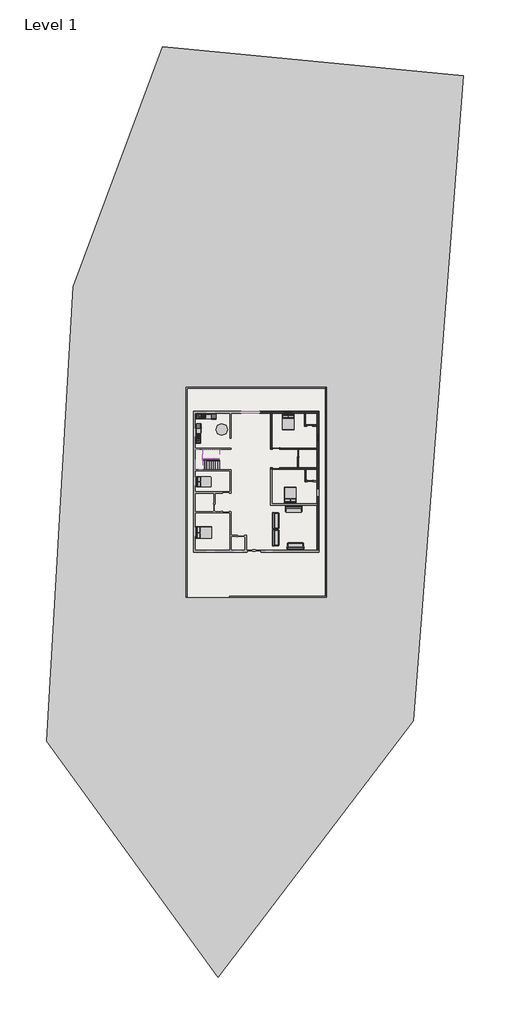
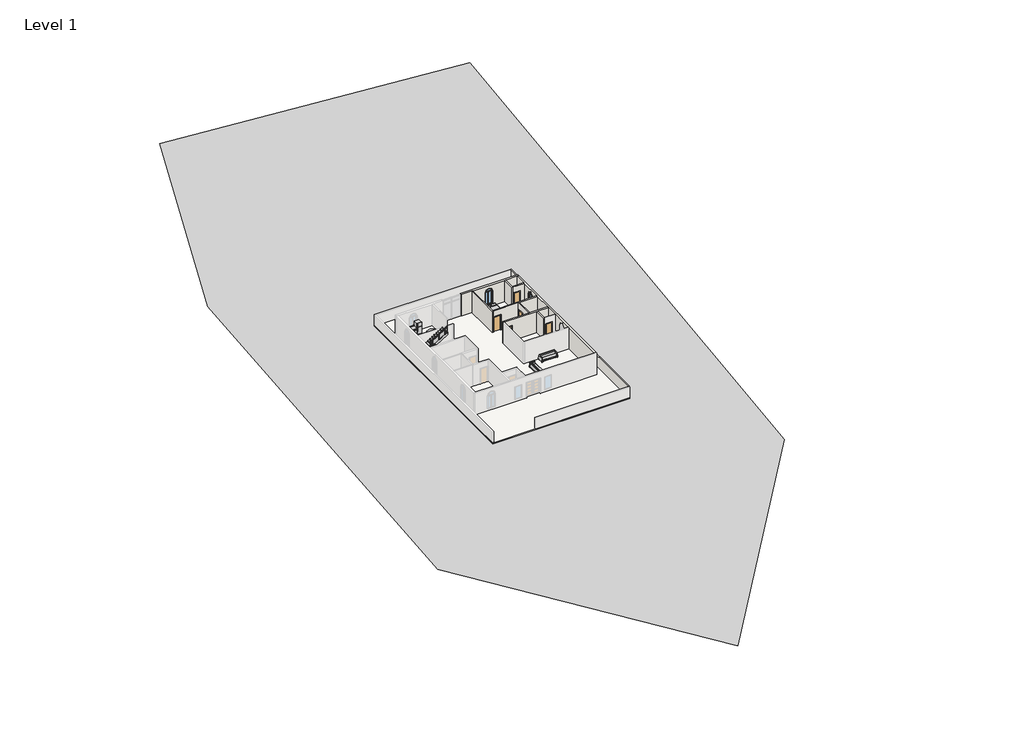
# One storey, part 2 of 2: 11 furniture elements, 10 walls, 9 proxies, 5 doors, 3 members, 2 flow terminals, 2 slabs, 2 stair flights, 3 other elements.
"""IFC4 building model written with IfcOpenShell, lengths in millimetres."""

from ifc_helpers import new_model, si_unit, frame, origin, place, context, project, spatial, polyline, circle_curve, outline, extrude, faceted_brep, triangles, transform, mapped, element, save
from ifc_brep_helpers import plane_surface, revolved_surface, advanced_brep
from components import proxy_a6faaae8, proxy_45b28599, kitchenette_medium_kitchenette_medium_844211aa, proxy_c523a7b7, single_flush_2_5_e2b13fe9, door_686f89d2, door_16372e1c, flow_terminal_871c2e40, furniture_c8abb964, furniture_1d2926bd, furniture_c6510c7c, furniture_aff9b2fb, furniture_bbcc68ce, non_monolithic_landing_a6573d81, stair_flight_969e3d78, stair_flight_057ca7f5, window_e7489165

model = new_model("IFC4")

# Units and contexts
model_context = context("Model", 3, world=origin())
ifc_project = project(units=[si_unit("LENGTHUNIT", "METRE", prefix="MILLI")], contexts=[model_context])

# Site, building, storey
site = spatial("IfcSite", under=ifc_project)
building = spatial("IfcBuilding", under=site)
storey = spatial("IfcBuildingStorey", under=building, Name="Level 1", Elevation=0.0)

# Proxies
placement = place(None, origin())
element("IfcBuildingElementProxy", 1, Name="Building Element Proxy", at=placement, inside=storey, context=model_context, shape_type="Tessellation", body=[
    triangles([(-13362.1157867, 60522.4871704, -152.4), (26139.3672729, 56668.527063, -152.4), (19592.1599304, -27911.1312195, -152.4), (-6089.9317657, -61567.0048096, -152.4), (-28593.0151794, -30596.776593, -152.4), (-25067.8233765, 29048.3780823, -152.4)], [[6, 2, 1], [3, 6, 5], [3, 2, 6], [3, 5, 4]], closed=False),
])
proxy_shape = proxy_a6faaae8(model_context)
element("IfcBuildingElementProxy", 2, Name="Cook Top-4 Unit2 : 22\" x 20\"", ObjectType="Cook Top-4 Unit2 : 22\" x 20\"", at=placement, inside=storey, context=model_context, shape_type="MappedRepresentation", body=[
    mapped(proxy_shape, transform((-8593.9791271, 12037.2953048, 0.0), x_axis=(1.0, 0.0, 0.0), y_axis=(0.0, 1.0, 0.0), z_axis=(0.0, 0.0, 1.0))),
])
element("IfcBuildingElementProxy", 3, Name="Cook Top-4 Unit2 : 22\" x 20\"", ObjectType="Cook Top-4 Unit2 : 22\" x 20\"", at=placement, inside=storey, context=model_context, shape_type="MappedRepresentation", body=[
    mapped(proxy_shape, transform((-8670.1791271, 8836.8953048, 0.0), x_axis=(0.0, 1.0000000000000002, 0.0), y_axis=(-1.0000000000000002, 0.0, 0.0), z_axis=(0.0, 0.0, 1.0))),
])
proxy_2_shape = proxy_45b28599(model_context)
element("IfcBuildingElementProxy", 4, Name="Dishwasher : 24\" x 24\" x 34\"", ObjectType="Dishwasher : 24\" x 24\" x 34\"", at=placement, inside=storey, context=model_context, shape_type="MappedRepresentation", body=[
    mapped(proxy_2_shape, transform((-7642.7965956, 11745.44574, 0.0), x_axis=(1.0, 0.0, 0.0), y_axis=(0.0, 1.0, 0.0), z_axis=(0.0, 0.0, 1.0))),
])
element("IfcBuildingElementProxy", 5, Name="Dishwasher : 24\" x 24\" x 34\"", ObjectType="Dishwasher : 24\" x 24\" x 34\"", at=placement, inside=storey, context=model_context, shape_type="MappedRepresentation", body=[
    mapped(proxy_2_shape, transform((-8378.3295623, 9788.0778363, 0.0), x_axis=(0.0, 1.0000000000000002, 0.0), y_axis=(-1.0000000000000002, 0.0, 0.0), z_axis=(0.0, 0.0, 1.0))),
])
kitchenette_medium_kitchenette_medium_shape = kitchenette_medium_kitchenette_medium_844211aa(model_context)
element("IfcBuildingElementProxy", 6, Name="Kitchenette - Medium : Kitchenette - Medium", ObjectType="Kitchenette - Medium : Kitchenette - Medium", at=placement, inside=storey, context=model_context, shape_type="MappedRepresentation", body=[
    mapped(kitchenette_medium_kitchenette_medium_shape, transform((-8269.816832, 12342.0953048, 0.0), x_axis=(1.0, 0.0, 0.0), y_axis=(0.0, 1.0, 0.0), z_axis=(0.0, 0.0, 1.0))),
])
element("IfcBuildingElementProxy", 7, Name="Kitchenette - Medium : Kitchenette - Medium", ObjectType="Kitchenette - Medium : Kitchenette - Medium", at=placement, inside=storey, context=model_context, shape_type="MappedRepresentation", body=[
    mapped(kitchenette_medium_kitchenette_medium_shape, transform((-8974.9791271, 9161.0575999, 0.0), x_axis=(0.0, 1.0000000000000002, 0.0), y_axis=(-1.0000000000000002, 0.0, 0.0), z_axis=(0.0, 0.0, 1.0))),
])
proxy_3_shape = proxy_c523a7b7(model_context)
element("IfcBuildingElementProxy", 8, Name="Refrigerator : 24\" x 25\" LH", ObjectType="Refrigerator : 24\" x 25\" LH", at=placement, inside=storey, context=model_context, shape_type="MappedRepresentation", body=[
    mapped(proxy_3_shape, transform((-6657.2291271, 11991.6463333, 0.0), x_axis=(1.0, 0.0, 0.0), y_axis=(0.0, 1.0, 0.0), z_axis=(0.0, 0.0, 1.0))),
])
element("IfcBuildingElementProxy", 9, Name="Refrigerator : 24\" x 25\" LH", ObjectType="Refrigerator : 24\" x 25\" LH", at=placement, inside=storey, context=model_context, shape_type="MappedRepresentation", body=[
    mapped(proxy_3_shape, transform((-8624.5301556, 10773.6453048, 0.0), x_axis=(0.0, 1.0000000000000002, 0.0), y_axis=(-1.0000000000000002, 0.0, 0.0), z_axis=(0.0, 0.0, 1.0))),
])

# Doors
single_flush_2_5_shape = single_flush_2_5_e2b13fe9(model_context)
element("IfcDoor", 10, ObjectType="Single-Flush : 2.5'", at=placement, inside=storey, context=model_context, shape_type="MappedRepresentation", body=[
    mapped(single_flush_2_5_shape, transform((6023.7208729, 3515.5953048, 0.0), x_axis=(-1.0, 0.0, 0.0), y_axis=(0.0, -1.0, 0.0), z_axis=(0.0, 0.0, 1.0))),
])
element("IfcDoor", 11, ObjectType="Single-Flush : 2.5'", at=placement, inside=storey, context=model_context, shape_type="MappedRepresentation", body=[
    mapped(single_flush_2_5_shape, transform((5947.5208729, 10830.7953048, 0.0), x_axis=(-1.0, 0.0, 0.0), y_axis=(0.0, -1.0, 0.0), z_axis=(0.0, 0.0, 1.0))),
])
door_shape = door_686f89d2(model_context)
element("IfcDoor", 12, ObjectType="Single-Flush : 36\" x 84\"", at=placement, inside=storey, context=model_context, shape_type="MappedRepresentation", body=[
    mapped(door_shape, transform((1527.9208729, 7782.7953048, 0.0), x_axis=(-1.0, 0.0, 0.0), y_axis=(0.0, -1.0, 0.0), z_axis=(0.0, 0.0, 1.0))),
])
element("IfcDoor", 13, ObjectType="Single-Flush : 36\" x 84\"", at=placement, inside=storey, context=model_context, shape_type="MappedRepresentation", body=[
    mapped(door_shape, transform((4423.5208729, 7173.1953048, 0.0), x_axis=(0.0, 1.0, 0.0), y_axis=(-1.0, 0.0, 0.0), z_axis=(0.0, 0.0, 1.0))),
])
door_2_shape = door_16372e1c(model_context)
element("IfcDoor", 14, ObjectType="Single-Flush : 36\" x 84\"", at=placement, inside=storey, context=model_context, shape_type="MappedRepresentation", body=[
    mapped(door_2_shape, transform((1527.9208729, 5191.9953048, 0.0), x_axis=(-1.0, 0.0, 0.0), y_axis=(0.0, -1.0, 0.0), z_axis=(0.0, 0.0, 1.0))),
])

# Flow terminals
flow_terminal_shape = flow_terminal_871c2e40(model_context)
element("IfcFlowTerminal", 15, ObjectType="Sink Kitchen-Island : 18\" x 18\"", at=placement, inside=storey, context=model_context, shape_type="MappedRepresentation", body=[
    mapped(flow_terminal_shape, transform((-7936.5683676, 12034.9499037, -14.4), x_axis=(1.0, 0.0, 0.0), y_axis=(0.0, 1.0, 0.0), z_axis=(0.0, 0.0, 1.0))),
])
element("IfcFlowTerminal", 16, ObjectType="Sink Kitchen-Island : 18\" x 18\"", at=placement, inside=storey, context=model_context, shape_type="MappedRepresentation", body=[
    mapped(flow_terminal_shape, transform((-8667.833726, 9494.3060642, -14.4), x_axis=(0.0, 1.0000000000000002, 0.0), y_axis=(-1.0000000000000002, 0.0, 0.0), z_axis=(0.0, 0.0, 1.0))),
])

# Furniture
furniture_shape = furniture_c8abb964(model_context)
element("IfcFurniture", 17, ObjectType="Bed-Box : Double 53\" x 74\"", at=placement, inside=storey, context=model_context, shape_type="MappedRepresentation", body=[
    mapped(furniture_shape, transform((-8168.0086353, 3100.2428458, 0.0), x_axis=(0.0, 1.0, 0.0), y_axis=(-1.0, 0.0, 0.0), z_axis=(0.0, 0.0, 1.0))),
])
furniture_2_shape = furniture_1d2926bd(model_context)
element("IfcFurniture", 18, ObjectType="Bed-Box : Queen 60\" x 79\"", at=placement, inside=storey, context=model_context, shape_type="MappedRepresentation", body=[
    mapped(furniture_2_shape, transform((-8168.0086353, -3571.0046952, 0.0), x_axis=(0.0, 1.0000000000000002, 0.0), y_axis=(-1.0000000000000002, 0.0, 0.0), z_axis=(0.0, 0.0, 1.0))),
])
element("IfcFurniture", 19, ObjectType="Bed-Box : Queen 60\" x 79\"", at=placement, inside=storey, context=model_context, shape_type="MappedRepresentation", body=[
    mapped(furniture_2_shape, transform((3759.3733319, 1477.7657966, 0.0), x_axis=(-1.0, 0.0, 0.0), y_axis=(0.0, -1.0, 0.0), z_axis=(0.0, 0.0, 1.0))),
])
element("IfcFurniture", 20, ObjectType="Bed-Box : Queen 60\" x 79\"", at=placement, inside=storey, context=model_context, shape_type="MappedRepresentation", body=[
    mapped(furniture_2_shape, transform((2801.6684139, 11535.124813, 0.0), x_axis=(1.0000000000000002, 0.0, 0.0), y_axis=(0.0, 1.0000000000000002, 0.0), z_axis=(0.0, 0.0, 1.0))),
])
furniture_3_shape = furniture_c6510c7c(model_context)
element("IfcFurniture", 21, ObjectType="Counter Top w Sink Hole : 24\" Depth", at=placement, inside=storey, context=model_context, shape_type="MappedRepresentation", body=[
    mapped(furniture_3_shape, transform((-7736.416832, 12342.0953048, -14.4), x_axis=(1.0, 0.0, 0.0), y_axis=(0.0, 1.0, 0.0), z_axis=(0.0, 0.0, 1.0))),
])
element("IfcFurniture", 22, ObjectType="Counter Top w Sink Hole : 24\" Depth", at=placement, inside=storey, context=model_context, shape_type="MappedRepresentation", body=[
    mapped(furniture_3_shape, transform((-8974.9791271, 9694.4575999, -14.4), x_axis=(0.0, 1.0000000000000002, 0.0), y_axis=(-1.0000000000000002, 0.0, 0.0), z_axis=(0.0, 0.0, 1.0))),
])
furniture_4_shape = furniture_aff9b2fb(model_context)
element("IfcFurniture", 23, ObjectType="Sofa-Pensi : 84\"", at=placement, inside=storey, context=model_context, shape_type="MappedRepresentation", body=[
    mapped(furniture_4_shape, transform((3586.1146229, -419.1145313, 0.0), x_axis=(1.0, 0.0, 0.0), y_axis=(0.0, 1.0, 0.0), z_axis=(0.0, 0.0, 1.0))),
])
element("IfcFurniture", 24, ObjectType="Sofa-Pensi : 84\"", at=placement, inside=storey, context=model_context, shape_type="MappedRepresentation", body=[
    mapped(furniture_4_shape, transform((1754.230709, -1944.6109452, 0.0), x_axis=(0.0, 1.0000000000000002, 0.0), y_axis=(-1.0000000000000002, 0.0, 0.0), z_axis=(0.0, 0.0, 1.0))),
])
element("IfcFurniture", 25, ObjectType="Sofa-Pensi : 84\"", at=placement, inside=storey, context=model_context, shape_type="MappedRepresentation", body=[
    mapped(furniture_4_shape, transform((4371.9271229, -4728.9948591, 0.0), x_axis=(-1.0000000000000004, 0.0, 0.0), y_axis=(0.0, -1.0000000000000004, 0.0), z_axis=(0.0, 0.0, 1.0))),
])
element("IfcFurniture", 26, ObjectType="Sofa-Pensi : 84\"", at=placement, inside=storey, context=model_context, shape_type="MappedRepresentation", body=[
    mapped(furniture_4_shape, transform((1754.230709, -4179.8109452, 0.0), x_axis=(0.0, 1.0000000000000009, 0.0), y_axis=(-1.0000000000000009, 0.0, 0.0), z_axis=(0.0, 0.0, 1.0))),
])
furniture_5_shape = furniture_bbcc68ce(model_context)
element("IfcFurniture", 27, ObjectType="Table-Dining Round w Chairs : 36\" Diameter", at=placement, inside=storey, context=model_context, shape_type="MappedRepresentation", body=[
    mapped(furniture_5_shape, transform((-5687.7610943, 10482.2739933, 0.0), x_axis=(1.0, 0.0, 0.0), y_axis=(0.0, 1.0, 0.0), z_axis=(0.0, 0.0, 1.0))),
])

# Members
element("IfcMember", 28, ObjectType="Stringer - 2\" Width", at=placement, inside=storey, context=model_context, shape_type="SweptSolid", body=[
    extrude(outline(polyline([(0.0, -5888.8791271), (215.0106437, -5888.8791271), (1605.083371, -8073.2791271), (1243.8010268, -8073.2791271), (0.0, -6118.7346564), (0.0, -5888.8791271)])), frame((0.0, 6233.3953048, 0.0), z_axis=(0.0, 1.0, 0.0), x_axis=(0.0, 0.0, 1.0)), (0.0, 0.0, 1.0), 50.8),
])
element("IfcMember", 29, ObjectType="Stringer - 2\" Width", at=placement, inside=storey, context=model_context, shape_type="SweptSolid", body=[
    extrude(outline(polyline([(1815.2106437, -8124.0791271), (1453.9282995, -8124.0791271), (2876.3282995, -5888.8791271), (3237.6106437, -5888.8791271), (1815.2106437, -8124.0791271)])), frame((0.0, 6411.1953048, 0.0), z_axis=(0.0, 1.0, 0.0), x_axis=(0.0, 0.0, 1.0)), (0.0, 0.0, 1.0), 50.8),
])
element("IfcMember", 30, ObjectType="Stringer - 2\" Width", at=placement, inside=storey, context=model_context, shape_type="SweptSolid", body=[
    extrude(outline(polyline([(-8073.2791271, 6233.3953048), (-8124.0791271, 6233.3953048), (-8124.0791271, 6411.1953048), (-8073.2791271, 6411.1953048), (-8073.2791271, 6233.3953048)])), frame((0.0, 0.0, 1371.6), z_axis=(0.0, 0.0, 1.0), x_axis=(1.0, 0.0, 0.0)), (0.0, 0.0, 1.0), 304.8),
])

# Railing
element("IfcRailing", 31, ObjectType="Glass Panel - Bottom Fill", at=placement, inside=storey, context=model_context, shape_type="SolidModel", body=[
    faceted_brep([(-5888.8791271, 6182.5953048, 1092.2), (-5888.8791271, 6182.5953048, 1031.986276), (-5888.8791271, 6233.3953048, 1031.986276), (-5888.8791271, 6233.3953048, 1092.2), (-8047.8791271, 6182.5953048, 2466.1090909), (-8098.6791271, 6182.5953048, 2438.2226396), (-8098.6791271, 6233.3953048, 2438.2226396), (-8047.8791271, 6233.3953048, 2466.1090909), (-8174.8791271, 6309.5953048, 2463.8), (-8174.8791271, 6309.5953048, 2514.6), (-8174.8791271, 6385.7953048, 2514.6), (-8174.8791271, 6436.5953048, 2463.8), (-8124.0791271, 6309.5953048, 2463.8), (-8124.0791271, 6436.5953048, 2463.8), (-8124.0791271, 6309.5953048, 2514.6), (-8124.0791271, 6385.7953048, 2514.6), (-8174.8791271, 6385.7953048, 2740.8909091), (-8174.8791271, 6436.5953048, 2690.0909091), (-8124.0791271, 6436.5953048, 2690.0909091), (-8124.0791271, 6385.7953048, 2740.8909091), (-5888.8791271, 6512.7953048, 4114.8), (-5888.8791271, 6461.9953048, 4114.8), (-5888.8791271, 6461.9953048, 4054.586276), (-5888.8791271, 6512.7953048, 4054.586276), (-8033.0861322, 6512.7953048, 2690.0909091), (-8047.8791271, 6512.7953048, 2740.8909091), (-8033.0861322, 6461.9953048, 2690.0909091), (-8047.8791271, 6461.9953048, 2740.8909091), (-8047.8791271, 6182.5953048, 2514.6), (-8098.6791271, 6182.5953048, 2463.8), (-8098.6791271, 6233.3953048, 2463.8), (-8047.8791271, 6233.3953048, 2514.6), (-8174.8791271, 6182.5953048, 2514.6), (-8174.8791271, 6182.5953048, 2463.8), (-8124.0791271, 6233.3953048, 2463.8), (-8124.0791271, 6233.3953048, 2514.6), (-8174.8791271, 6512.7953048, 2740.8909091), (-8174.8791271, 6512.7953048, 2690.0909091), (-8124.0791271, 6461.9953048, 2690.0909091), (-8124.0791271, 6461.9953048, 2740.8909091)], [[[0, 1, 2, 3]], [[1, 0, 4, 5]], [[2, 1, 5, 6]], [[3, 2, 6, 7]], [[0, 3, 7, 4]], [[8, 9, 10, 11]], [[12, 8, 11, 13]], [[14, 12, 13, 15]], [[9, 14, 15, 10]], [[11, 10, 16, 17]], [[13, 11, 17, 18]], [[15, 13, 18, 19]], [[10, 15, 19, 16]], [[20, 21, 22, 23]], [[24, 25, 20, 23]], [[26, 24, 23, 22]], [[27, 26, 22, 21]], [[25, 27, 21, 20]], [[5, 4, 28, 29]], [[6, 5, 29, 30]], [[7, 6, 30, 31]], [[4, 7, 31, 28]], [[29, 28, 32, 33]], [[30, 29, 33, 34]], [[31, 30, 34, 35]], [[28, 31, 35, 32]], [[33, 32, 9, 8]], [[34, 33, 8, 12]], [[35, 34, 12, 14]], [[32, 35, 14, 9]], [[17, 16, 36, 37]], [[18, 17, 37, 38]], [[19, 18, 38, 39]], [[16, 19, 39, 36]], [[37, 36, 25, 24]], [[38, 37, 24, 26]], [[39, 38, 26, 27]], [[36, 39, 27, 25]]]),
    faceted_brep([(-5888.8791271, 6220.6953048, 1005.653431), (-5888.8791271, 6195.2953048, 1005.653431), (-5888.8791271, 6195.2953048, 975.546569), (-5888.8791271, 6220.6953048, 975.546569), (-8120.3808784, 6220.6953048, 2425.7), (-8120.3808784, 6195.2953048, 2425.7), (-8127.7773758, 6195.2953048, 2400.3), (-8127.7773758, 6220.6953048, 2400.3), (-8136.7791271, 6220.6953048, 2425.7), (-8162.1791271, 6195.2953048, 2425.7), (-8162.1791271, 6195.2953048, 2400.3), (-8136.7791271, 6220.6953048, 2400.3), (-8136.7791271, 6474.6953048, 2425.7), (-8136.7791271, 6474.6953048, 2400.3), (-8162.1791271, 6474.6953048, 2400.3), (-8162.1791271, 6474.6953048, 2425.7)], [[[0, 1, 2, 3]], [[1, 0, 4, 5]], [[2, 1, 5, 6]], [[3, 2, 6, 7]], [[0, 3, 7, 4]], [[5, 4, 8, 9]], [[6, 5, 9, 10]], [[7, 6, 10, 11]], [[4, 7, 11, 8]], [[12, 13, 14, 15]], [[9, 8, 12, 15]], [[10, 9, 15, 14]], [[11, 10, 14, 13]], [[8, 11, 13, 12]]]),
    faceted_brep([(-8162.1791271, 6474.6953048, 2581.6079765), (-8162.1791271, 6500.0953048, 2581.6079765), (-8162.1791271, 6500.0953048, 2551.5011144), (-8162.1791271, 6474.6953048, 2551.5011144), (-5888.8791271, 6474.6953048, 4028.253431), (-5888.8791271, 6474.6953048, 3998.146569), (-5888.8791271, 6500.0953048, 3998.146569), (-5888.8791271, 6500.0953048, 4028.253431)], [[[0, 1, 2, 3]], [[4, 5, 6, 7]], [[1, 0, 4, 7]], [[2, 1, 7, 6]], [[3, 2, 6, 5]], [[0, 3, 5, 4]]]),
    faceted_brep([(-5888.8791271, 6220.6953048, 904.053431), (-5888.8791271, 6195.2953048, 904.053431), (-5888.8791271, 6195.2953048, 873.946569), (-5888.8791271, 6220.6953048, 873.946569), (-8120.3808784, 6220.6953048, 2324.1), (-8120.3808784, 6195.2953048, 2324.1), (-8127.7773758, 6195.2953048, 2298.7), (-8127.7773758, 6220.6953048, 2298.7), (-8136.7791271, 6220.6953048, 2324.1), (-8162.1791271, 6195.2953048, 2324.1), (-8162.1791271, 6195.2953048, 2298.7), (-8136.7791271, 6220.6953048, 2298.7), (-8136.7791271, 6474.6953048, 2324.1), (-8136.7791271, 6474.6953048, 2298.7), (-8162.1791271, 6474.6953048, 2298.7), (-8162.1791271, 6474.6953048, 2324.1)], [[[0, 1, 2, 3]], [[1, 0, 4, 5]], [[2, 1, 5, 6]], [[3, 2, 6, 7]], [[0, 3, 7, 4]], [[5, 4, 8, 9]], [[6, 5, 9, 10]], [[7, 6, 10, 11]], [[4, 7, 11, 8]], [[12, 13, 14, 15]], [[9, 8, 12, 15]], [[10, 9, 15, 14]], [[11, 10, 14, 13]], [[8, 11, 13, 12]]]),
    faceted_brep([(-8162.1791271, 6474.6953048, 2480.0079765), (-8162.1791271, 6500.0953048, 2480.0079765), (-8162.1791271, 6500.0953048, 2449.9011144), (-8162.1791271, 6474.6953048, 2449.9011144), (-5888.8791271, 6474.6953048, 3926.653431), (-5888.8791271, 6474.6953048, 3896.546569), (-5888.8791271, 6500.0953048, 3896.546569), (-5888.8791271, 6500.0953048, 3926.653431)], [[[0, 1, 2, 3]], [[4, 5, 6, 7]], [[1, 0, 4, 7]], [[2, 1, 7, 6]], [[3, 2, 6, 5]], [[0, 3, 5, 4]]]),
    extrude(outline(polyline([(3856.5817305, -6200.0291271), (3848.4999123, -6212.7291271), (2844.8, -6212.7291271), (2844.8, -6200.0291271), (3856.5817305, -6200.0291271)])), frame((0.0, 6461.9953048, 0.0), z_axis=(0.0, 1.0, 0.0), x_axis=(0.0, 0.0, 1.0)), (0.0, 0.0, 1.0), 50.8),
    extrude(outline(polyline([(2509.9818182, -7019.1791271), (3027.2181818, -6206.3791271), (3694.5011144, -6206.3791271), (3177.2647508, -7019.1791271), (2509.9818182, -7019.1791271)])), frame((0.0, 6487.5804618, 0.0), z_axis=(0.0, 1.0, 0.0), x_axis=(0.0, 0.0, 1.0)), (0.0, 0.0, 1.0), 6.35),
    extrude(outline(polyline([(3339.3453669, -7012.8291271), (3331.2635487, -7025.5291271), (2311.4, -7025.5291271), (2311.4, -7012.8291271), (3339.3453669, -7012.8291271)])), frame((0.0, 6461.9953048, 0.0), z_axis=(0.0, 1.0, 0.0), x_axis=(0.0, 0.0, 1.0)), (0.0, 0.0, 1.0), 50.8),
    extrude(outline(polyline([(1976.5818182, -7831.9791271), (2493.8181818, -7019.1791271), (3177.2647508, -7019.1791271), (2660.0283872, -7831.9791271), (1976.5818182, -7831.9791271)])), frame((0.0, 6487.5804618, 0.0), z_axis=(0.0, 1.0, 0.0), x_axis=(0.0, 0.0, 1.0)), (0.0, 0.0, 1.0), 6.35),
    extrude(outline(polyline([(2822.1090032, -7825.6291271), (2814.0271851, -7838.3291271), (1955.8, -7838.3291271), (1955.8, -7825.6291271), (2822.1090032, -7825.6291271)])), frame((0.0, 6461.9953048, 0.0), z_axis=(0.0, 1.0, 0.0), x_axis=(0.0, 0.0, 1.0)), (0.0, 0.0, 1.0), 50.8),
    extrude(outline(polyline([(2256.3817305, -7812.9291271), (2264.4635487, -7825.6291271), (1244.6, -7825.6291271), (1244.6, -7812.9291271), (2256.3817305, -7812.9291271)])), frame((0.0, 6182.5953048, 0.0), z_axis=(0.0, 1.0, 0.0), x_axis=(0.0, 0.0, 1.0)), (0.0, 0.0, 1.0), 50.8),
    extrude(outline(polyline([(909.7818182, -7006.4791271), (1585.146569, -7006.4791271), (2102.3829326, -7819.2791271), (1427.0181818, -7819.2791271), (909.7818182, -7006.4791271)])), frame((0.0, 6201.4601478, 0.0), z_axis=(0.0, 1.0, 0.0), x_axis=(0.0, 0.0, 1.0)), (0.0, 0.0, 1.0), 6.35),
    extrude(outline(polyline([(1739.1453669, -7000.1291271), (1747.2271851, -7012.8291271), (889.0, -7012.8291271), (889.0, -7000.1291271), (1739.1453669, -7000.1291271)])), frame((0.0, 6182.5953048, 0.0), z_axis=(0.0, 1.0, 0.0), x_axis=(0.0, 0.0, 1.0)), (0.0, 0.0, 1.0), 50.8),
    extrude(outline(polyline([(376.3818182, -6193.6791271), (1067.9102054, -6193.6791271), (1585.146569, -7006.4791271), (893.6181818, -7006.4791271), (376.3818182, -6193.6791271)])), frame((0.0, 6201.4601478, 0.0), z_axis=(0.0, 1.0, 0.0), x_axis=(0.0, 0.0, 1.0)), (0.0, 0.0, 1.0), 6.35),
    extrude(outline(polyline([(1221.9090032, -6187.3291271), (1229.9908214, -6200.0291271), (355.6, -6200.0291271), (355.6, -6187.3291271), (1221.9090032, -6187.3291271)])), frame((0.0, 6182.5953048, 0.0), z_axis=(0.0, 1.0, 0.0), x_axis=(0.0, 0.0, 1.0)), (0.0, 0.0, 1.0), 50.8),
    extrude(outline(polyline([(-8159.0041271, 6477.8703048), (-8159.0041271, 6496.9203048), (-8139.9541271, 6496.9203048), (-8139.9541271, 6477.8703048), (-8159.0041271, 6477.8703048)])), frame((0.0, 0.0, 1600.2), z_axis=(0.0, 0.0, 1.0), x_axis=(1.0, 0.0, 0.0)), (0.0, 0.0, 1.0), 1089.8909091),
    extrude(outline(polyline([(-8139.9541271, 6217.5203048), (-8139.9541271, 6198.4703048), (-8159.0041271, 6198.4703048), (-8159.0041271, 6217.5203048), (-8139.9541271, 6217.5203048)])), frame((0.0, 0.0, 1600.2), z_axis=(0.0, 0.0, 1.0), x_axis=(1.0, 0.0, 0.0)), (0.0, 0.0, 1.0), 863.6),
    extrude(outline(polyline([(-8114.5541271, 6217.5203048), (-8114.5541271, 6198.4703048), (-8133.6041271, 6198.4703048), (-8133.6041271, 6217.5203048), (-8114.5541271, 6217.5203048)])), frame((0.0, 0.0, 1600.2), z_axis=(0.0, 0.0, 1.0), x_axis=(1.0, 0.0, 0.0)), (0.0, 0.0, 1.0), 863.6),
    extrude(outline(polyline([(4058.6271851, -5882.5291271), (4046.5044578, -5901.5791271), (3022.6, -5901.5791271), (3022.6, -5882.5291271), (4058.6271851, -5882.5291271)])), frame((0.0, 6477.8703048, 0.0), z_axis=(0.0, 1.0, 0.0), x_axis=(0.0, 0.0, 1.0)), (0.0, 0.0, 1.0), 19.05),
    extrude(outline(polyline([(1027.9453669, -5882.5291271), (1040.0680941, -5901.5791271), (177.8, -5901.5791271), (177.8, -5882.5291271), (1027.9453669, -5882.5291271)])), frame((0.0, 6198.4703048, 0.0), z_axis=(0.0, 1.0, 0.0), x_axis=(0.0, 0.0, 1.0)), (0.0, 0.0, 1.0), 19.05),
])

# Slabs
element("IfcSlab", 32, ObjectType="6\"", at=placement, inside=storey, context=model_context, shape_type="SweptSolid", body=[
    extrude(outline(polyline([(8157.3208729, 15859.9953048), (8157.3208729, -11724.4046952), (-10283.0791271, -11724.4046952), (-10283.0791271, 15859.9953048), (8157.3208729, 15859.9953048)])), frame((0.0, 0.0, -152.4), z_axis=(0.0, 0.0, 1.0), x_axis=(1.0, 0.0, 0.0)), (0.0, 0.0, 1.0), 152.4),
])
non_monolithic_landing_shape = non_monolithic_landing_a6573d81(model_context)
element("IfcSlab", 33, ObjectType="Non-Monolithic Landing", at=placement, inside=storey, context=model_context, shape_type="MappedRepresentation", body=[
    mapped(non_monolithic_landing_shape, transform((0.0, 0.0, 0.0), x_axis=(1.0, 0.0, 0.0), y_axis=(0.0, 1.0, 0.0), z_axis=(0.0, 0.0, 1.0))),
])

# Stair flights
stair_flight_shape = stair_flight_969e3d78(model_context)
element("IfcStairFlight", 34, ObjectType="2\" Tread 1\" Nosing 1/4\" Riser", at=placement, inside=storey, context=model_context, shape_type="MappedRepresentation", body=[
    mapped(stair_flight_shape, transform((0.0, 0.0, 0.0), x_axis=(1.0, 0.0, 0.0), y_axis=(0.0, 1.0, 0.0), z_axis=(0.0, 0.0, 1.0))),
])
stair_flight_2_shape = stair_flight_057ca7f5(model_context)
element("IfcStairFlight", 35, ObjectType="2\" Tread 1\" Nosing 1/4\" Riser", at=placement, inside=storey, context=model_context, shape_type="MappedRepresentation", body=[
    mapped(stair_flight_2_shape, transform((0.0, 0.0, 0.0), x_axis=(1.0, 0.0, 0.0), y_axis=(0.0, 1.0, 0.0), z_axis=(0.0, 0.0, 1.0))),
])

# Walls
element("IfcWall", 36, ObjectType="6\"", at=placement, inside=storey, context=model_context, shape_type="Brep", body=[
    faceted_brep([(8004.9208729, 15859.9953048, 0.0), (8004.9208729, 15707.5953048, 0.0), (8004.9208729, -11572.0046952, 0.0), (8004.9208729, -11572.0046952, 1524.0), (8004.9208729, 15707.5953048, 1524.0), (8004.9208729, 15859.9953048, 1524.0), (8157.3208729, 15859.9953048, 0.0), (8157.3208729, 15859.9953048, 1524.0), (8157.3208729, -11572.0046952, 1524.0), (8157.3208729, -11572.0046952, 0.0)], [[[0, 1, 2, 3, 4, 5]], [[6, 7, 8, 9]], [[2, 1, 0, 6, 9]], [[5, 4, 3, 8, 7]], [[0, 5, 7, 6]], [[3, 2, 9, 8]]]),
])
element("IfcWall", 37, ObjectType="6\"", at=placement, inside=storey, context=model_context, shape_type="Brep", body=[
    faceted_brep([(842.1208729, 12430.9953048, 0.0), (842.1208729, 7706.5953048, 0.0), (842.1208729, 7706.5953048, 3048.0), (842.1208729, 12430.9953048, 3048.0), (994.5208729, 12430.9953048, 0.0), (994.5208729, 12430.9953048, 3048.0), (994.5208729, 7858.9953048, 3048.0), (994.5208729, 7706.5953048, 3048.0), (994.5208729, 7706.5953048, 0.0), (994.5208729, 7858.9953048, 0.0)], [[[0, 1, 2, 3]], [[4, 5, 6, 7, 8, 9]], [[1, 0, 4, 9, 8]], [[3, 2, 7, 6, 5]], [[0, 3, 5, 4]], [[2, 1, 8, 7]]]),
])
element("IfcWall", 38, ObjectType="6\"", at=placement, inside=storey, context=model_context, shape_type="Brep", body=[
    faceted_brep([(994.5208729, 7706.5953048, 0.0), (1070.7208729, 7706.5953048, 0.0), (1070.7208729, 7706.5953048, 2133.6), (1985.1208729, 7706.5953048, 2133.6), (1985.1208729, 7706.5953048, 0.0), (4347.3208729, 7706.5953048, 0.0), (4499.7208729, 7706.5953048, 0.0), (6938.1208729, 7706.5953048, 0.0), (6938.1208729, 7706.5953048, 3048.0), (4499.7208729, 7706.5953048, 3048.0), (4347.3208729, 7706.5953048, 3048.0), (994.5208729, 7706.5953048, 3048.0), (1070.7208729, 7858.9953048, 2133.6), (1070.7208729, 7858.9953048, 0.0), (994.5208729, 7858.9953048, 0.0), (994.5208729, 7858.9953048, 3048.0), (6938.1208729, 7858.9953048, 3048.0), (6938.1208729, 7858.9953048, 0.0), (1985.1208729, 7858.9953048, 0.0), (1985.1208729, 7858.9953048, 2133.6)], [[[0, 1, 2, 3, 4, 5, 6, 7, 8, 9, 10, 11]], [[12, 13, 14, 15, 16, 17, 18, 19]], [[18, 17, 7, 6, 5, 4]], [[14, 13, 1, 0]], [[11, 10, 9, 8, 16, 15]], [[0, 11, 15, 14]], [[8, 7, 17, 16]], [[2, 1, 13, 12]], [[3, 2, 12, 19]], [[4, 3, 19, 18]]]),
])
element("IfcWall", 39, ObjectType="6\"", at=placement, inside=storey, context=model_context, shape_type="Brep", body=[
    faceted_brep([(1070.7208729, 5268.1953048, 2133.6), (1070.7208729, 5268.1953048, 0.0), (842.1208729, 5268.1953048, 0.0), (842.1208729, 5268.1953048, 3048.0), (4347.3208729, 5268.1953048, 3048.0), (4499.7208729, 5268.1953048, 3048.0), (6938.1208729, 5268.1953048, 3048.0), (6938.1208729, 5268.1953048, 0.0), (4499.7208729, 5268.1953048, 0.0), (4347.3208729, 5268.1953048, 0.0), (1985.1208729, 5268.1953048, 0.0), (1985.1208729, 5268.1953048, 2133.6), (842.1208729, 5115.7953048, 0.0), (994.5208729, 5115.7953048, 0.0), (1070.7208729, 5115.7953048, 0.0), (1070.7208729, 5115.7953048, 2133.6), (1985.1208729, 5115.7953048, 2133.6), (1985.1208729, 5115.7953048, 0.0), (5337.9208729, 5115.7953048, 0.0), (5490.3208729, 5115.7953048, 0.0), (6938.1208729, 5115.7953048, 0.0), (6938.1208729, 5115.7953048, 3048.0), (5490.3208729, 5115.7953048, 3048.0), (5337.9208729, 5115.7953048, 3048.0), (994.5208729, 5115.7953048, 3048.0), (842.1208729, 5115.7953048, 3048.0)], [[[0, 1, 2, 3, 4, 5, 6, 7, 8, 9, 10, 11]], [[12, 13, 14, 15, 16, 17, 18, 19, 20, 21, 22, 23, 24, 25]], [[2, 1, 14, 13, 12]], [[10, 9, 8, 7, 20, 19, 18, 17]], [[6, 5, 4, 3, 25, 24, 23, 22, 21]], [[7, 6, 21, 20]], [[3, 2, 12, 25]], [[15, 14, 1, 0]], [[16, 15, 0, 11]], [[17, 16, 11, 10]]]),
])
element("IfcWall", 40, ObjectType="6\"", at=placement, inside=storey, context=model_context, shape_type="SweptSolid", body=[
    extrude(outline(polyline([(7706.5953048, 0.0), (7630.3953048, 0.0), (7630.3953048, 2133.6), (6715.9953048, 2133.6), (6715.9953048, 0.0), (5268.1953048, 0.0), (5268.1953048, 3048.0), (7706.5953048, 3048.0), (7706.5953048, 0.0)])), frame((4347.3208729, 0.0, 0.0), z_axis=(1.0, 0.0, 0.0), x_axis=(0.0, 1.0, 0.0)), (0.0, 0.0, 1.0), 152.4),
])
element("IfcWall", 41, ObjectType="6\"", at=placement, inside=storey, context=model_context, shape_type="Brep", body=[
    faceted_brep([(5261.7208729, 12430.9953048, 0.0), (5261.7208729, 10754.5953048, 0.0), (5261.7208729, 10754.5953048, 3048.0), (5261.7208729, 12430.9953048, 3048.0), (5414.1208729, 12430.9953048, 0.0), (5414.1208729, 12430.9953048, 3048.0), (5414.1208729, 10906.9953048, 3048.0), (5414.1208729, 10754.5953048, 3048.0), (5414.1208729, 10754.5953048, 0.0), (5414.1208729, 10906.9953048, 0.0)], [[[0, 1, 2, 3]], [[4, 5, 6, 7, 8, 9]], [[1, 0, 4, 9, 8]], [[3, 2, 7, 6, 5]], [[0, 3, 5, 4]], [[2, 1, 8, 7]]]),
])
element("IfcWall", 42, ObjectType="6\"", at=placement, inside=storey, context=model_context, shape_type="SweptSolid", body=[
    extrude(outline(polyline([(0.0, 5414.1208729), (0.0, 5566.5208729), (2133.6, 5566.5208729), (2133.6, 6328.5208729), (0.0, 6328.5208729), (0.0, 6938.1208729), (3048.0, 6938.1208729), (3048.0, 5414.1208729), (0.0, 5414.1208729)])), frame((0.0, 10754.5953048, 0.0), z_axis=(0.0, 1.0, 0.0), x_axis=(0.0, 0.0, 1.0)), (0.0, 0.0, 1.0), 152.4),
])
element("IfcWall", 43, ObjectType="6\"", at=placement, inside=storey, context=model_context, shape_type="Brep", body=[
    faceted_brep([(5337.9208729, 5115.7953048, 0.0), (5337.9208729, 3439.3953048, 0.0), (5337.9208729, 3439.3953048, 3048.0), (5337.9208729, 5115.7953048, 3048.0), (5490.3208729, 5115.7953048, 0.0), (5490.3208729, 5115.7953048, 3048.0), (5490.3208729, 3591.7953048, 3048.0), (5490.3208729, 3439.3953048, 3048.0), (5490.3208729, 3439.3953048, 0.0), (5490.3208729, 3591.7953048, 0.0)], [[[0, 1, 2, 3]], [[4, 5, 6, 7, 8, 9]], [[1, 0, 4, 9, 8]], [[3, 2, 7, 6, 5]], [[0, 3, 5, 4]], [[2, 1, 8, 7]]]),
])
element("IfcWall", 44, ObjectType="9\"", at=placement, inside=storey, context=model_context, shape_type="AdvancedBrep", body=[
    advanced_brep(
    [(6938.1208729, 12430.9953048, 0.0), (6938.1208729, 10906.9953048, 0.0), (6938.1208729, 10754.5953048, 0.0), (6938.1208729, 7858.9953048, 0.0), (6938.1208729, 7706.5953048, 0.0), (6938.1208729, 5268.1953048, 0.0), (6938.1208729, 5115.7953048, 0.0), (6938.1208729, 3591.7953048, 0.0), (6938.1208729, 3439.3953048, 0.0), (6938.1208729, 543.7953048, 0.0), (6938.1208729, 391.3953048, 0.0), (6938.1208729, -5552.2046952, 0.0), (6938.1208729, -5552.2046952, 3048.0), (6938.1208729, 391.3953048, 3048.0), (6938.1208729, 543.7953048, 3048.0), (6938.1208729, 3439.3953048, 3048.0), (6938.1208729, 3591.7953048, 3048.0), (6938.1208729, 5115.7953048, 3048.0), (6938.1208729, 5268.1953048, 3048.0), (6938.1208729, 7706.5953048, 3048.0), (6938.1208729, 7858.9953048, 3048.0), (6938.1208729, 10754.5953048, 3048.0), (6938.1208729, 10906.9953048, 3048.0), (6938.1208729, 12430.9953048, 3048.0), (6938.1208729, 8849.5953048, 2152.65), (6938.1208729, 8849.5953048, 304.8), (6938.1208729, 9763.9953048, 304.8), (6938.1208729, 9763.9953048, 2152.65), (6938.1208729, 1534.3953048, 2152.65), (6938.1208729, 1534.3953048, 304.8), (6938.1208729, 2448.7953048, 304.8), (6938.1208729, 2448.7953048, 2152.65), (7166.7208729, 12430.9953048, 0.0), (7166.7208729, 12430.9953048, 3048.0), (7166.7208729, -5552.2046952, 3048.0), (7166.7208729, -5552.2046952, 0.0), (7166.7208729, 8849.5953048, 2152.65), (7166.7208729, 9763.9953048, 2152.65), (7166.7208729, 9763.9953048, 304.8), (7166.7208729, 8849.5953048, 304.8), (7166.7208729, 1534.3953048, 2152.65), (7166.7208729, 2448.7953048, 2152.65), (7166.7208729, 2448.7953048, 304.8), (7166.7208729, 1534.3953048, 304.8)],
    [
        (0, 1),
        (1, 2),
        (2, 3),
        (3, 4),
        (4, 5),
        (5, 6),
        (6, 7),
        (7, 8),
        (8, 9),
        (9, 10),
        (10, 11),
        (11, 12),
        (12, 13),
        (13, 14),
        (14, 15),
        (15, 16),
        (16, 17),
        (17, 18),
        (18, 19),
        (19, 20),
        (20, 21),
        (21, 22),
        (22, 23),
        (23, 0),
        (24, 25),
        (25, 26),
        (26, 27),
        (27, 24, circle_curve(frame((6938.1208729, 9306.7953048, 2152.65), z_axis=(1.0, 0.0, 0.0), x_axis=(0.0, -1.0, 0.0)), 457.2)),
        (28, 29),
        (29, 30),
        (30, 31),
        (31, 28, circle_curve(frame((6938.1208729, 1991.5953048, 2152.65), z_axis=(1.0, 0.0, 0.0), x_axis=(0.0, -1.0, 0.0)), 457.2)),
        (32, 33),
        (33, 34),
        (34, 35),
        (35, 32),
        (36, 37, circle_curve(frame((7166.7208729, 9306.7953048, 2152.65), z_axis=(-1.0, 0.0, 0.0), x_axis=(0.0, -1.0, 0.0)), 457.2)),
        (37, 38),
        (38, 39),
        (39, 36),
        (40, 41, circle_curve(frame((7166.7208729, 1991.5953048, 2152.65), z_axis=(-1.0, 0.0, 0.0), x_axis=(0.0, -1.0, 0.0)), 457.2)),
        (41, 42),
        (42, 43),
        (43, 40),
        (0, 32),
        (35, 11),
        (12, 34),
        (33, 23),
        (24, 36),
        (39, 25),
        (38, 26),
        (37, 27),
        (28, 40),
        (43, 29),
        (42, 30),
        (41, 31),
    ],
    [
        plane_surface(frame((6938.1208729, 12430.9953048, 0.0), z_axis=(-1.0, 0.0, 0.0), x_axis=(0.0, -1.0, 0.0))),
        plane_surface(frame((7166.7208729, 12430.9953048, 0.0), z_axis=(1.0, 0.0, 0.0), x_axis=(0.0, 1.0, 0.0))),
        plane_surface(frame((6938.1208729, 12545.2953048, 0.0), z_axis=(0.0, 0.0, -1.0), x_axis=(1.0, 0.0, 0.0))),
        plane_surface(frame((6938.1208729, -5666.5046952, 3048.0), z_axis=(0.0, 0.0, 1.0), x_axis=(1.0, 0.0, 0.0))),
        plane_surface(frame((-10130.6791271, 12430.9953048, 0.0), z_axis=(0.0, 1.0, 0.0), x_axis=(1.0, 0.0, 0.0))),
        plane_surface(frame((-10130.6791271, -5552.2046952, 0.0), z_axis=(0.0, -1.0, 0.0), x_axis=(-1.0, 0.0, 0.0))),
        plane_surface(frame((6938.1208729, 8849.5953048, 2152.65), z_axis=(0.0, 1.0, 0.0), x_axis=(1.0, 0.0, 0.0))),
        plane_surface(frame((6938.1208729, 8849.5953048, 304.8), z_axis=(0.0, 0.0, 1.0), x_axis=(1.0, 0.0, 0.0))),
        plane_surface(frame((6938.1208729, 9763.9953048, 304.8), z_axis=(0.0, -1.0, 0.0), x_axis=(1.0, 0.0, 0.0))),
        revolved_surface(polyline([(7166.7208729, 8849.5953048, 2152.65), (6938.1208729, 8849.5953048, 2152.65)]), (6938.1208729, 9306.7953048, 2152.65), (1.0, 0.0, 0.0)),
        plane_surface(frame((6938.1208729, 1534.3953048, 2152.65), z_axis=(0.0, 1.0, 0.0), x_axis=(1.0, 0.0, 0.0))),
        plane_surface(frame((6938.1208729, 1534.3953048, 304.8), z_axis=(0.0, 0.0, 1.0), x_axis=(1.0, 0.0, 0.0))),
        plane_surface(frame((6938.1208729, 2448.7953048, 304.8), z_axis=(0.0, -1.0, 0.0), x_axis=(1.0, 0.0, 0.0))),
        revolved_surface(polyline([(7166.7208729, 1534.3953047999998, 2152.65), (6938.1208729, 1534.3953047999998, 2152.65)]), (6938.1208729, 1991.5953048, 2152.65), (1.0, 0.0, 0.0)),
    ],
    [
        (0, [[1, 2, 3, 4, 5, 6, 7, 8, 9, 10, 11, 12, 13, 14, 15, 16, 17, 18, 19, 20, 21, 22, 23, 24], [25, 26, 27, 28], [29, 30, 31, 32]]),
        (1, [[33, 34, 35, 36], [37, 38, 39, 40], [41, 42, 43, 44]]),
        (2, [[-11, -10, -9, -8, -7, -6, -5, -4, -3, -2, -1, 45, -36, 46]]),
        (3, [[-23, -22, -21, -20, -19, -18, -17, -16, -15, -14, -13, 47, -34, 48]]),
        (4, [[-24, -48, -33, -45]]),
        (5, [[-12, -46, -35, -47]]),
        (6, [[-25, 49, -40, 50]]),
        (7, [[-26, -50, -39, 51]]),
        (8, [[-27, -51, -38, 52]]),
        (9, [[-28, -52, -37, -49]]),
        (10, [[-29, 53, -44, 54]]),
        (11, [[-30, -54, -43, 55]]),
        (12, [[-31, -55, -42, 56]]),
        (13, [[-32, -56, -41, -53]]),
    ],
),
])
element("IfcWall", 45, ObjectType="9\"", at=placement, inside=storey, context=model_context, shape_type="AdvancedBrep", body=[
    advanced_brep(
    [(-605.6791271, 12430.9953048, 0.0), (842.1208729, 12430.9953048, 0.0), (994.5208729, 12430.9953048, 0.0), (5261.7208729, 12430.9953048, 0.0), (5414.1208729, 12430.9953048, 0.0), (6938.1208729, 12430.9953048, 0.0), (7166.7208729, 12430.9953048, 0.0), (7166.7208729, 12430.9953048, 3048.0), (6938.1208729, 12430.9953048, 3048.0), (5414.1208729, 12430.9953048, 3048.0), (5261.7208729, 12430.9953048, 3048.0), (994.5208729, 12430.9953048, 3048.0), (842.1208729, 12430.9953048, 3048.0), (-605.6791271, 12430.9953048, 3048.0), (3585.3208729, 12430.9953048, 2152.65), (3585.3208729, 12430.9953048, 304.8), (2670.9208729, 12430.9953048, 304.8), (2670.9208729, 12430.9953048, 2152.65), (-605.6791271, 12659.5953048, 0.0), (-605.6791271, 12659.5953048, 3048.0), (7166.7208729, 12659.5953048, 3048.0), (7166.7208729, 12659.5953048, 0.0), (3585.3208729, 12659.5953048, 2152.65), (2670.9208729, 12659.5953048, 2152.65), (2670.9208729, 12659.5953048, 304.8), (3585.3208729, 12659.5953048, 304.8)],
    [
        (0, 1),
        (1, 2),
        (2, 3),
        (3, 4),
        (4, 5),
        (5, 6),
        (6, 7),
        (7, 8),
        (8, 9),
        (9, 10),
        (10, 11),
        (11, 12),
        (12, 13),
        (13, 0),
        (14, 15),
        (15, 16),
        (16, 17),
        (17, 14, circle_curve(frame((3128.1208729, 12430.9953048, 2152.65), z_axis=(0.0, 1.0, 0.0), x_axis=(1.0, 0.0, 0.0)), 457.2)),
        (18, 19),
        (19, 20),
        (20, 21),
        (21, 18),
        (22, 23, circle_curve(frame((3128.1208729, 12659.5953048, 2152.65), z_axis=(0.0, -1.0, 0.0), x_axis=(1.0, 0.0, 0.0)), 457.2)),
        (23, 24),
        (24, 25),
        (25, 22),
        (0, 18),
        (21, 6),
        (20, 7),
        (19, 13),
        (17, 23),
        (22, 14),
        (25, 15),
        (24, 16),
    ],
    [
        plane_surface(frame((-10130.6791271, 12430.9953048, 0.0), z_axis=(0.0, -1.0, 0.0), x_axis=(1.0, 0.0, 0.0))),
        plane_surface(frame((-10130.6791271, 12659.5953048, 0.0), z_axis=(0.0, 1.0, 0.0), x_axis=(-1.0, 0.0, 0.0))),
        plane_surface(frame((-605.6791271, 12430.9953048, 0.0), z_axis=(0.0, 0.0, -1.0), x_axis=(0.0, 1.0, 0.0))),
        plane_surface(frame((7166.7208729, 12430.9953048, 0.0), z_axis=(1.0, 0.0, 0.0), x_axis=(0.0, 1.0, 0.0))),
        plane_surface(frame((7166.7208729, 12430.9953048, 3048.0), z_axis=(0.0, 0.0, 1.0), x_axis=(0.0, 1.0, 0.0))),
        plane_surface(frame((-605.6791271, 12430.9953048, 3048.0), z_axis=(-1.0, 0.0, 0.0), x_axis=(0.0, 1.0, 0.0))),
        revolved_surface(polyline([(3585.3208729, 12659.5953048, 2152.65), (3585.3208729, 12430.9953048, 2152.65)]), (3128.1208729, 12430.9953048, 2152.65), (0.0, 1.0, 0.0)),
        plane_surface(frame((3585.3208729, 12430.9953048, 2152.65), z_axis=(-1.0, 0.0, 0.0), x_axis=(0.0, 1.0, 0.0))),
        plane_surface(frame((3585.3208729, 12430.9953048, 304.8), z_axis=(0.0, 0.0, 1.0), x_axis=(0.0, 1.0, 0.0))),
        plane_surface(frame((2670.9208729, 12430.9953048, 304.8), z_axis=(1.0, 0.0, 0.0), x_axis=(0.0, 1.0, 0.0))),
    ],
    [
        (0, [[1, 2, 3, 4, 5, 6, 7, 8, 9, 10, 11, 12, 13, 14], [15, 16, 17, 18]]),
        (1, [[19, 20, 21, 22], [23, 24, 25, 26]]),
        (2, [[-6, -5, -4, -3, -2, -1, 27, -22, 28]]),
        (3, [[-7, -28, -21, 29]]),
        (4, [[-13, -12, -11, -10, -9, -8, -29, -20, 30]]),
        (5, [[-14, -30, -19, -27]]),
        (6, [[-18, 31, -23, 32]]),
        (7, [[-15, -32, -26, 33]]),
        (8, [[-16, -33, -25, 34]]),
        (9, [[-17, -34, -24, -31]]),
    ],
),
])

# Windows
window_shape = window_e7489165(model_context)
element("IfcWindow", 46, ObjectType="36\" x 72\"", at=placement, inside=storey, context=model_context, shape_type="MappedRepresentation", body=[
    mapped(window_shape, transform((3120.1187148, 12545.2953048, 0.0), x_axis=(1.0, 0.0, 0.0), y_axis=(0.0, 1.0, 0.0), z_axis=(0.0, 0.0, 1.0))),
])
element("IfcWindow", 47, ObjectType="36\" x 72\"", at=placement, inside=storey, context=model_context, shape_type="MappedRepresentation", body=[
    mapped(window_shape, transform((7052.4208729, 9314.7974629, 0.0), x_axis=(0.0, -1.0, 0.0), y_axis=(1.0, 0.0, 0.0), z_axis=(0.0, 0.0, 1.0))),
])

save(model, "model.ifc")

# Revit data of these elements
# Type "Cook Top-4 Unit2 : 22\" x 20\""
#   Depth = 1' - 8"
#   Width = 1' - 10"
#   Burner Material = Steel, Chrome Plated
#   Cooktop Material = Steel, Polished
#   Default Elevation = 0
#   Assembly Code = ""
# Type "Dishwasher : 24\" x 24\" x 34\""
#   Label = "DW"
#   Assembly Code = "E1090400"
#   Depth = 2' - 0"
#   Height = 2' - 10"
#   Width = 2' - 0"
#   Dishwasher Material = Steel, Paint Finish, Ivory, Glossy
#   Panel Face Material = Plastic, Opaque Black
#   Default Elevation = 0
# Type "Kitchenette - Medium : Kitchenette - Medium"
#   Assembly Code = "E1090400"
#   Counter Length = 6' - 6"
#   Cabinet Width = 4' - 6"
#   Cabinet Height = 2' - 10 1/2"
#   Cabinet Depth = 2' - 0"
#   Toe Depth = 0' - 3"
#   Toe Height = 0' - 3 1/2"
#   Cabinet Material = Cabinets
#   Door/Drawer Material = Cabinets
#   Handle Material = Cabinets - Handles
#   Default Elevation = 0
# Type "Refrigerator : 24\" x 25\" LH"
#   Label = "REF."
#   Assembly Code = "E1090400"
#   Depth = 2' - 0 3/4"
#   Handle = 0' - 1 1/2"
#   Height = 5' - 3 1/2"
#   Rear Clearance = 0' - 2"
#   Top Door Height = 1' - 8"
#   Width = 1' - 11 1/2"
#   Material = Steel, Paint Finish, Ivory, Glossy
#   Default Elevation = 0
# Type "Single-Flush : 2.5'"
#   Type Mark = "8"
#   Construction Type Id = "MDOOR"
#   Assembly Code = "C1020"
#   Analytic Construction = "Metal"
#   Thickness = 0' - 2"
#   Heat Transfer Coefficient (U) = 0.651978 BTU/(h·ft²·°F)
#   Height = 7' - 0"
#   Trim Projection Ext = 0' - 1"
#   Trim Projection Int = 0' - 1"
#   Trim Width = 0' - 3"
#   Width = 2' - 6"
#   Define Thermal Properties by = 1
#   Door Material = Door - Panel
#   Frame Material = Door - Frame
#   Visual Light Transmittance = 0
#   Solar Heat Gain Coefficient = 0
#   Function = (empty or 0)
#   Wall Closure = (empty or 0)
# Type "Single-Flush : 36\" x 84\""
#   Type Mark = "1"
#   Construction Type Id = "MDOOR"
#   Assembly Code = "C1020"
#   Analytic Construction = "Metal"
#   Thickness = 0' - 2"
#   Heat Transfer Coefficient (U) = 0.651978 BTU/(h·ft²·°F)
#   Height = 7' - 0"
#   Trim Projection Ext = 0' - 1"
#   Trim Projection Int = 0' - 1"
#   Trim Width = 0' - 3"
#   Width = 3' - 0"
#   Define Thermal Properties by = 1
#   Door Material = Door - Panel
#   Frame Material = Door - Frame
#   Visual Light Transmittance = 0
#   Solar Heat Gain Coefficient = 0
#   Function = (empty or 0)
#   Wall Closure = (empty or 0)
# Type "Sink Kitchen-Island : 18\" x 18\""
#   Assembly Code = "D2010410"
#   Counter Height = 3' - 0"
#   Depth = 1' - 6"
#   Width = 1' - 6"
#   Faucet Material = Steel, Polished
#   Sink Material = Steel, Polished
#   Default Elevation = 0
# Type "Bed-Box : Double 53\" x 74\""
#   Assembly Code = "E2020200"
#   Length = 6' - 2"
#   Width = 4' - 5"
#   Frame Material = Birch
#   Mattress Material = Linen, White
#   Default Elevation = 0
# Type "Bed-Box : Queen 60\" x 79\""
#   Assembly Code = "E2020200"
#   Length = 6' - 7"
#   Width = 5' - 0"
#   Frame Material = Birch
#   Mattress Material = Linen, White
#   Default Elevation = 0
# Type "Counter Top w Sink Hole : 24\" Depth"
#   Assembly Code = "C1030400"
#   Counter Thickness = 0' - 1 1/2"
#   Depth = 2' - 1"
#   Height = 3' - 0"
#   Length [instance default] = 8' - 0"
#   Sink Location [instance default] = 2' - 0"
#   Sink Location To Wall [instance default] = 0' - 6"
#   Sink Opening Depth [instance default] = 1' - 3"
#   Sink Opening Width [instance default] = 2' - 3"
#   Counter Top Material = none
#   Default Elevation = 0
# Type "Sofa-Pensi : 84\""
#   Assembly Code = "E2020200"
#   Length = 7' - 0"
#   Frame Material = Cherry
#   Seat Material = Linen, Beige
#   Feet Material = Steel, Chrome Plated
#   Default Elevation = 0
# Type "Table-Dining Round w Chairs : 36\" Diameter"
#   Assembly Code = "E2020200"
#   Radius = 2' - 6"
#   Diameter = 5' - 0"
#   Height = 2' - 6"
#   Chairs = 8
#   Base Material = Pine
#   Top Material = Laminate, Linen, Matte
#   Default Elevation = 0
# Type "Glass Panel - Bottom Fill"
#   Assembly Code = "C2010400"
#   built-in parameter 1008612 = 0.0416667 (stored number, unit not read)
#   built-in parameter 1008611 = 0.0416667 (stored number, unit not read)
#   built-in parameter 1008609 = 0.333333 (stored number, unit not read)
#   built-in parameter 1008604 = 0.166667 (stored number, unit not read)
#   built-in parameter 1008603 = 0.166667 (stored number, unit not read)
#   Railing Height = 3' - 0"
#   built-in parameter 1008630 = 2
#   built-in parameter 1008610 = 2
#   built-in parameter 1008618 = Baluster - Square : 3/4"
# Type "6\""
#   Assembly Code = "B1010"
#   Function = 0
#   Layers, outside or top first: 0' - 6" "FLOOR" (function 1)
# Type "6\""
#   Assembly Code = "B2010"
#   Layers, outside or top first: 0' - 6" "INT WALL" (function 1)
# Type "9\""
#   Assembly Code = "B2010"
#   Layers, outside or top first: 0' - 9" "EXT WALL" (function 1)
# Type "36\" x 72\""
#   Type Mark = "10"
#   Construction Type Id = "SGL"
#   Assembly Code = "B2020100"
#   Analytic Construction = "Large single-glazed windows"
#   Visual Light Transmittance = 0.9
#   Solar Heat Gain Coefficient = 0.86
#   Heat Transfer Coefficient (U) = 0.979472 BTU/(h·ft²·°F)
#   Height = 6' - 0"
#   Default Sill Height = 1' - 0"
#   Trim Projection - Ext. = 0' - 0 1/2"
#   Trim Projection - Int. = 0' - 0 3/4"
#   Trim Width - Exterior = 0' - 3 1/2"
#   Trim Width - Interior = 0' - 3 1/2"
#   Width = 3' - 0"
#   Window Inset = 0' - 0 3/4"
#   Define Thermal Properties by = 1
#   Glass Pane Material = Glass
#   Sash Material = Sash
#   Trim Exterior Material = Trim
#   Trim Interior Material = Trim
#   Wall Closure = (empty or 0)
# Element 1 (IfcBuildingElementProxy)
#   Material = GRASS
#   Phase Created = New Construction
# Elements 2, 3 (IfcBuildingElementProxy, "Cook Top-4 Unit2 : 22\" x 20\"")
#   Phase Created = New Construction
#   Materials on its faces: "Steel, Chrome Plated", "Steel, Polished"
# Elements 4, 5 (IfcBuildingElementProxy, "Dishwasher : 24\" x 24\" x 34\"")
#   Phase Created = New Construction
#   Materials on its faces: "Steel, Paint Finish, Ivory, Glossy", "Plastic, Opaque Black"
# Elements 6, 7 (IfcBuildingElementProxy, "Kitchenette - Medium : Kitchenette - Medium")
#   Phase Created = New Construction
#   Materials on its faces: "Cabinets", "Cabinets - Handles"
# Elements 8, 9 (IfcBuildingElementProxy, "Refrigerator : 24\" x 25\" LH")
#   Phase Created = New Construction
#   Materials on its faces: "Steel, Paint Finish, Ivory, Glossy", "Steel, Chrome Plated"
# Elements 10, 11 (IfcDoor, "Single-Flush : 2.5'")
#   Phase Created = New Construction
#   Materials on its faces: "Door - Frame", "Door - Panel"
# Elements 12, 13, 14 (IfcDoor, "Single-Flush : 36\" x 84\"")
#   Phase Created = New Construction
#   Materials on its faces: "Door - Frame", "Door - Panel"
# Element 15 (IfcFlowTerminal, "Sink Kitchen-Island : 18\" x 18\"")
#   Mark = "1"
#   Phase Created = New Construction
#   Materials on its faces: "Steel, Polished"
# Element 16 (IfcFlowTerminal, "Sink Kitchen-Island : 18\" x 18\"")
#   Mark = "2"
#   Phase Created = New Construction
#   Materials on its faces: "Steel, Polished"
# Element 17 (IfcFurniture, "Bed-Box : Double 53\" x 74\"")
#   Phase Created = New Construction
#   Materials on its faces: "Birch", "Linen, White"
# Elements 18, 19, 20 (IfcFurniture, "Bed-Box : Queen 60\" x 79\"")
#   Phase Created = New Construction
#   Materials on its faces: "Birch", "Linen, White"
# Elements 21, 22 (IfcFurniture, "Counter Top w Sink Hole : 24\" Depth")
#   Sink Opening Depth = 1' - 2"
#   Sink Location To Wall = 0' - 6"
#   Length = 6' - 6"
#   Sink Location = 3' - 4"
#   Sink Opening Width = 1' - 4"
#   Phase Created = New Construction
#   Materials on its faces: "Counter Top"
# Elements 23, 24, 25, 26 (IfcFurniture, "Sofa-Pensi : 84\"")
#   Phase Created = New Construction
#   Materials on its faces: "Cherry", "Linen, Beige", "Steel, Chrome Plated"
# Element 27 (IfcFurniture, "Table-Dining Round w Chairs : 36\" Diameter")
#   Phase Created = New Construction
#   Materials on its faces: "Pine", "Laminate, Linen, Matte"
# Elements 28, 29, 30 (IfcMember, "Stringer - 2\" Width")
#   Phase Created = New Construction
# Element 31 (IfcRailing, "Glass Panel - Bottom Fill")
#   Phase Created = New Construction
#   Materials on its faces: "Glass"
# Element 32 (IfcSlab, "6\"")
#   Height Offset From Level = 0' - 0"
#   Phase Created = New Construction
#   Materials on its faces: "FLOOR"
# Element 33 (IfcSlab, "Non-Monolithic Landing")
#   Phase Created = New Construction
# Elements 34, 35 (IfcStairFlight, "2\" Tread 1\" Nosing 1/4\" Riser")
#   Phase Created = New Construction
# Element 36 (IfcWall, "6\"")
#   Top Offset = 0' - 0"
#   Base Offset = 0' - 0"
#   Unconnected Height = 5' - 0"
#   wall height = 5' - 0"
#   Phase Created = New Construction
#   Base Constraint = Level 1
#   Materials on its faces: "INT WALL"
# Elements 37, 38, 39, 40, 41, 42, 43 (IfcWall, "6\"")
#   Top Offset = 0' - 0"
#   Base Offset = 0' - 0"
#   Unconnected Height = 10' - 0"
#   wall height = 10' - 0"
#   Phase Created = New Construction
#   Base Constraint = Level 1
#   Materials on its faces: "INT WALL"
# Elements 44, 45 (IfcWall, "9\"")
#   Top Offset = 0' - 0"
#   Base Offset = 0' - 0"
#   Unconnected Height = 10' - 0"
#   wall height = 10' - 0"
#   Phase Created = New Construction
#   Base Constraint = Level 1
#   Materials on its faces: "EXT WALL"
# Element 46 (IfcWindow, "36\" x 72\"")
#   Mark = "8"
#   Phase Created = New Construction
#   Materials on its faces: "Sash", "Trim", "Glass"
# Element 47 (IfcWindow, "36\" x 72\"")
#   Mark = "9"
#   Phase Created = New Construction
#   Materials on its faces: "Sash", "Trim", "Glass"
# Materials
#   "Steel, Chrome Plated": class "Metal", colour RGB 17 17 17, transparency 0, Description = "Chromiuim plated steel", Cost = 0
#   "Steel, Polished": class "Metal", colour RGB 57 57 57, transparency 0, Description = "Polished steel", Cost = 0
#   "Steel, Paint Finish, Ivory, Glossy": class "Metal", colour RGB 247 247 239, transparency 0, Description = "Steel, paint finish, ivory, glossy", Cost = 0
#   "Plastic, Opaque Black": class "Plastic", colour RGB 0 0 0, transparency 0.7, Description = "Plastic, generic, opaque black", Cost = 0
#   "Cabinets": colour RGB 249 249 249, transparency 0
#   "Cabinets - Handles": class "Metal", colour RGB 57 57 57, transparency 0
#   "Door - Panel": class "Wood", colour RGB 210 159 95, transparency 0
#   "Door - Frame": colour RGB 118 70 51, transparency 0
#   "Birch": class "Wood", colour RGB 224 178 126, transparency 0, Description = "Betula Alleghaniensis", Cost = 0
#   "Linen, White": class "Textile", colour RGB 247 247 239, transparency 0, Description = "Linen, white", Cost = 0
#   "Cherry": class "Wood", colour RGB 226 177 128, transparency 0, Description = "Prunus Serotina", Cost = 0
#   "Linen, Beige": class "Textile", colour RGB 249 239 230, transparency 0, Description = "Linen, beige", Cost = 0
#   "Pine": class "Wood", colour RGB 223 192 134, transparency 0, Description = "Pinus Echinata", Cost = 0
#   "Laminate, Linen, Matte": class "Plastic", colour RGB 249 239 230, transparency 0, Description = "Plastic Laminate - Linen, Matte", Cost = 0
#   "FLOOR": class "Generic", colour RGB 140 134 116, transparency 0, Cost = 0
#   "INT WALL": class "Generic", colour RGB 164 133 98, transparency 0, Cost = 0
#   "EXT WALL": class "Generic", colour RGB 156 123 46, transparency 0, Cost = 0
#   "Glass": class "Glass", colour RGB 0 128 192, transparency 0.75, Description = "Soda Lime Glass", Cost = 0
#   "Sash": class "Wood", colour RGB 224 178 126, transparency 0
#   "Trim": class "Wood", colour RGB 224 178 126, transparency 0
#   "GRASS": class "Generic", colour RGB 127 136 91, transparency 0, Cost = 0
#   "Counter Top": class "Wood", colour RGB 226 177 128, transparency 0
